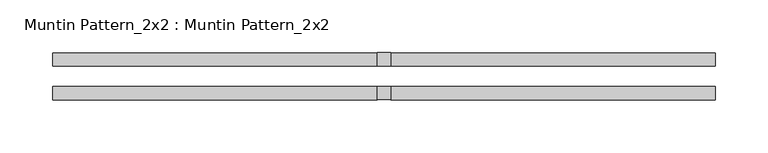
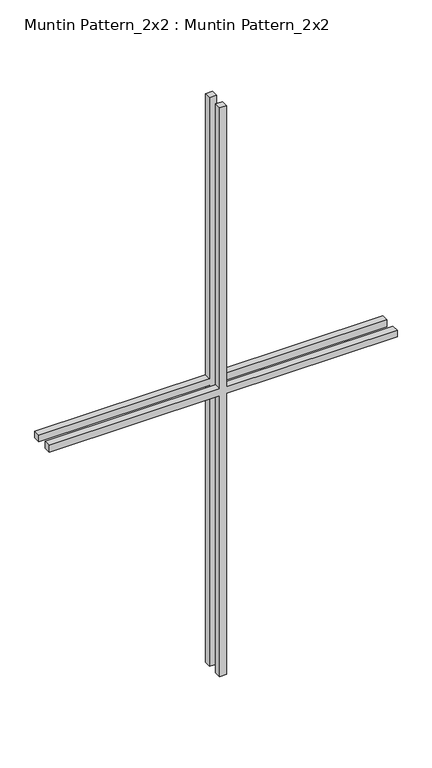
"""IFC4 building model written with IfcOpenShell, lengths in millimetres: proxy geometry, Muntin Pattern_2x2 : Muntin Pattern_2x2."""

from ifc_helpers import new_model, si_unit, frame, origin, place, context, project, spatial, polyline, outline, extrude, source, transform, mapped, element, save


def muntin_pattern_2x2_muntin_pattern_2x2_f598e128(model_context):
    return source(origin(), model_context, "Body", "SweptSolid", [
        extrude(outline(polyline([(546.1, -6.35), (546.1, -312.7375), (533.4, -312.7375), (533.4, -6.35), (0.0, -6.35), (0.0, 6.35), (533.4, 6.35), (533.4, 312.7375), (546.1, 312.7375), (546.1, 6.35), (1079.5, 6.35), (1079.5, -6.35), (546.1, -6.35)])), frame((0.0, -22.225, 0.0), z_axis=(0.0, 1.0, 0.0), x_axis=(0.0, 0.0, 1.0)), (0.0, 0.0, 1.0), 12.7),
        extrude(outline(polyline([(546.1, -6.35), (546.1, -312.7375), (533.4, -312.7375), (533.4, -6.35), (0.0, -6.35), (0.0, 6.35), (533.4, 6.35), (533.4, 312.7375), (546.1, 312.7375), (546.1, 6.35), (1079.5, 6.35), (1079.5, -6.35), (546.1, -6.35)])), frame((0.0, 9.525, 0.0), z_axis=(0.0, 1.0, 0.0), x_axis=(0.0, 0.0, 1.0)), (0.0, 0.0, 1.0), 12.7),
    ])


if __name__ == "__main__":
    model = new_model("IFC4")
    model_context = context("Model", 3, world=origin())
    ifc_project = project(units=[si_unit("LENGTHUNIT", "METRE", prefix="MILLI")], contexts=[model_context])
    site = spatial("IfcSite", under=ifc_project)
    building = spatial("IfcBuilding", under=site)
    placement = place(None, origin())
    muntin_pattern_2x2_muntin_pattern_2x2_shape = muntin_pattern_2x2_muntin_pattern_2x2_f598e128(model_context)
    element("IfcBuildingElementProxy", 1, Name="Muntin Pattern_2x2 : Muntin Pattern_2x2", ObjectType="Muntin Pattern_2x2 : Muntin Pattern_2x2", at=placement, inside=building, context=model_context, shape_type="MappedRepresentation", body=[
        mapped(muntin_pattern_2x2_muntin_pattern_2x2_shape, transform((0.0, 0.0, 0.0), x_axis=(1.0, 0.0, 0.0), y_axis=(0.0, 1.0, 0.0), z_axis=(0.0, 0.0, 1.0))),
    ])
    save(model, "model.ifc")

# Revit data of these elements
# Type "Muntin Pattern_2x2 : Muntin Pattern_2x2"
#   Width [instance default] = 4' - 0"
#   Thickness = 0' - 0 1/2"
#   Height [instance default] = 4' - 0"
#   Distance = 0' - 0 3/4"
#   Interior Material [instance default] = none
#   Exterior Material [instance default] = none
#   Default Elevation = 0
# Element 1 (IfcBuildingElementProxy, "Muntin Pattern_2x2 : Muntin Pattern_2x2")
#   Width = 2' - 0 5/8"
#   Height = 3' - 6 1/2"
#   Interior Material = Wood - Stained
#   Exterior Material = Clad - White
#   Materials on its faces: "Clad - White", "Wood - Stained"
# Materials
#   "Clad - White": class "Wood", colour RGB 242 242 238, transparency 0, Cost = 0
#   "Wood - Stained": class "Wood", colour RGB 224 178 126, transparency 0, Cost = 0
